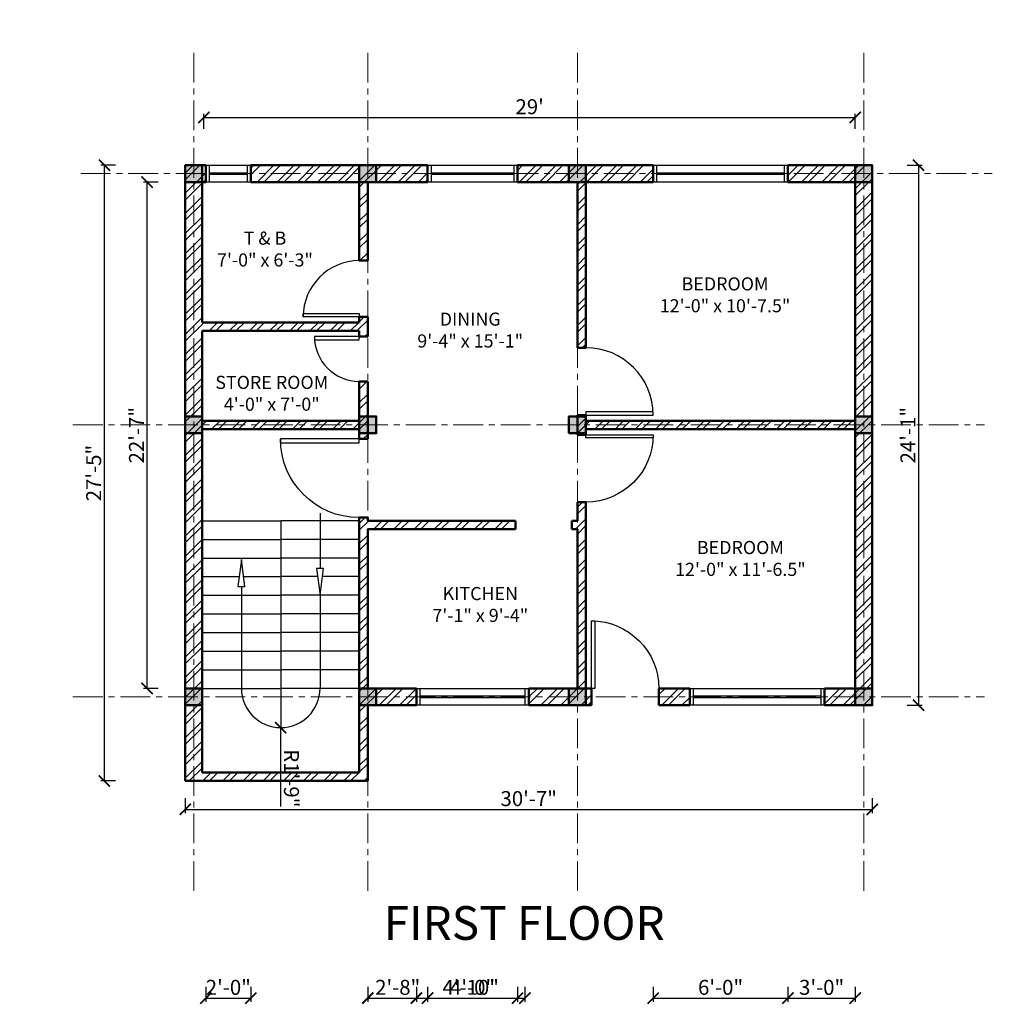
# Model space of a CAD drawing. Units: inches. Extents: x 378 to 1617, y 130 to 1256.
# Tile 4 of 5: x 1028 to 1548, y 134 to 660. Entities that reach past the tile are written whole.
import ezdxf

# ---------------------------------------------------------------- set-up
doc = ezdxf.new("R2010")
doc.units = ezdxf.units.IN
doc.linetypes.add('CENTER', pattern=[50.8, 31.75, -6.35, 6.35, -6.35])
for name, color, linetype, lineweight in [('A-ANNO-TEXT', 7, 'Continuous', 25), ('A-AREA-IDEN', 3, 'Continuous', 18), ('Column Hatch', 1, 'Continuous', 13), ('Columns', 241, 'Continuous', 50), ('Dimensions', 153, 'Continuous', 18), ('Doors', 2, 'Continuous', 25), ('Grid lines', 7, 'CENTER', 18), ('Stairs', 40, 'Continuous', 25), ('Wall Hatch', 11, 'Continuous', 13), ('Walls', 220, 'Continuous', 50), ('Windows', 140, 'Continuous', 25)]:
    doc.layers.add(name, color=color, linetype=linetype, lineweight=lineweight)
doc.styles.get("Standard").update_dxf_attribs({"font": 'arial.ttf'})
doc.dimstyles.new('ISO-25', dxfattribs={"dimtxt": 8, "dimasz": 6, "dimexe": 2, "dimexo": 4, "dimtad": 1, "dimdec": 0, "dimlunit": 3, "dimtxsty": 'Standard', "dimblk": 'ARCHTICK', "dimcen": 2.5, "dimadec": 0, "dimazin": 0, "dimtfac": 1, "dimtdec": 0, "dimtmove": 0, "dimatfit": 3, "dimfxl": 6, "dimfxlon": 1, "dimarcsym": 0})

# ---------------------------------------------------------------- blocks, each defined once
blk = doc.blocks.new('*U3')
for p, q in [((-30, 0), (-30, 4)), ((0, 0), (0, 4))]:
    blk.add_line(p, q)
blk.add_lwpolyline([(0, 0), (0, -30), (-1.75, -30), (-1.75, 0)], close=True)
blk.add_arc((0, 0), 30, 180, 270)
blk = doc.blocks.new('*U4')
for p, q in [((0, 0), (0, 4)), ((24, 0), (24, 4))]:
    blk.add_line(p, q)
blk.add_lwpolyline([(0, 0), (0, -24), (1.75, -24), (1.75, 0)], close=True)
blk.add_arc((0, 0), 24, 270, 0)
blk = doc.blocks.new('*U5')
for p, q in [((0, 0), (0, -4)), ((-36, 0), (-36, -4))]:
    blk.add_line(p, q)
blk.add_lwpolyline([(0, 0), (0, 36), (-1.75, 36), (-1.75, 0)], close=True)
blk.add_arc((0, 0), 36, 90, 180)
blk = doc.blocks.new('*U6')
for p, q in [((0, 0), (0, -4)), ((-36, 0), (-36, -4))]:
    blk.add_line(p, q)
blk.add_lwpolyline([(0, 0), (0, 36), (-1.75, 36), (-1.75, 0)], close=True)
blk.add_arc((0, 0), 36, 90, 180)
blk = doc.blocks.new('*U7')
for p, q in [((-36, 0), (-36, 4)), ((0, 0), (0, 4))]:
    blk.add_line(p, q)
blk.add_lwpolyline([(0, 0), (0, -36), (-1.75, -36), (-1.75, 0)], close=True)
blk.add_arc((0, 0), 36, 180, 270)
blk = doc.blocks.new('_ArchTick')
at = {"color": 0, "linetype": 'ByBlock', "const_width": 0.15}
blk.add_lwpolyline([(-0.5, -0.5), (0.5, 0.5)], dxfattribs=at)
blk = doc.blocks.new('*D39')
at = {"layer": 'Defpoints', "color": 0, "transparency": 16777216}
for p in [(1096.14, 572.95), (1125.53, 572.95), (1125.53, 302.45)]:
    blk.add_point(p, dxfattribs=at)
at = {"layer": 'Dimensions', "color": 0, "lineweight": -2, "transparency": 16777216}
for p, q in [((1102.14, 572.95), (1094.14, 572.95)), ((1096.14, 302.45), (1096.14, 572.95)), ((1102.14, 302.45), (1094.14, 302.45))]:
    blk.add_line(p, q, dxfattribs=at)
at = {"layer": 'Dimensions', "color": 0, "lineweight": -2, "transparency": 16777216, "xscale": 6, "yscale": 6, "zscale": 6}
for p, rotation in [((1096.14, 572.95), 90), ((1096.14, 302.45), 270)]:
    blk.add_blockref('_ArchTick', p, dxfattribs=dict(at, rotation=rotation))
at = {"layer": 'Dimensions', "color": 0, "transparency": 16777216, "insert": (1091.5, 437.7), "char_height": 8, "attachment_point": 5, "rotation": 90}
blk.add_mtext('22\'-7"', dxfattribs=at)
blk = doc.blocks.new('*D40')
at = {"layer": 'Defpoints', "color": 0, "transparency": 16777216}
for p in [(1474.53, 607.45), (1126.53, 572.95), (1474.53, 572.95)]:
    blk.add_point(p, dxfattribs=at)
at = {"layer": 'Dimensions', "color": 0, "lineweight": -2, "transparency": 16777216}
for p, q in [((1126.53, 601.45), (1126.53, 609.45)), ((1126.53, 607.45), (1474.53, 607.45)), ((1474.53, 601.45), (1474.53, 609.45))]:
    blk.add_line(p, q, dxfattribs=at)
at = {"layer": 'Dimensions', "color": 0, "lineweight": -2, "transparency": 16777216, "xscale": 6, "yscale": 6, "zscale": 6, "rotation": 180}
blk.add_blockref('_ArchTick', (1126.53, 607.45), dxfattribs=at)
at = {"layer": 'Dimensions', "color": 0, "lineweight": -2, "transparency": 16777216, "xscale": 6, "yscale": 6, "zscale": 6}
blk.add_blockref('_ArchTick', (1474.53, 607.45), dxfattribs=at)
at = {"layer": 'Dimensions', "color": 0, "transparency": 16777216, "insert": (1300.53, 612.16), "char_height": 8, "attachment_point": 5}
blk.add_mtext("29'", dxfattribs=at)
blk = doc.blocks.new('*D41')
at = {"layer": 'Defpoints', "color": 0, "transparency": 16777216}
for p in [(1483.53, 293.45), (1116.53, 252.95), (1483.53, 237.79)]:
    blk.add_point(p, dxfattribs=at)
at = {"layer": 'Dimensions', "color": 0, "lineweight": -2, "transparency": 16777216}
for p, q in [((1116.53, 243.79), (1116.53, 235.79)), ((1483.53, 243.79), (1483.53, 235.79)), ((1116.53, 237.79), (1483.53, 237.79))]:
    blk.add_line(p, q, dxfattribs=at)
at = {"layer": 'Dimensions', "color": 0, "lineweight": -2, "transparency": 16777216, "xscale": 6, "yscale": 6, "zscale": 6, "rotation": 180}
blk.add_blockref('_ArchTick', (1116.53, 237.79), dxfattribs=at)
at = {"layer": 'Dimensions', "color": 0, "lineweight": -2, "transparency": 16777216, "xscale": 6, "yscale": 6, "zscale": 6}
blk.add_blockref('_ArchTick', (1483.53, 237.79), dxfattribs=at)
at = {"layer": 'Dimensions', "color": 0, "transparency": 16777216, "insert": (1300.03, 242.5), "char_height": 8, "attachment_point": 5}
blk.add_mtext('30\'-7"', dxfattribs=at)
blk = doc.blocks.new('*D42')
at = {"layer": 'Defpoints', "color": 0, "transparency": 16777216}
for p in [(1073.34, 581.95), (1116.53, 581.95), (1116.53, 252.95)]:
    blk.add_point(p, dxfattribs=at)
at = {"layer": 'Dimensions', "color": 0, "lineweight": -2, "transparency": 16777216}
for p, q in [((1079.34, 581.95), (1071.34, 581.95)), ((1073.34, 252.95), (1073.34, 581.95)), ((1079.34, 252.95), (1071.34, 252.95))]:
    blk.add_line(p, q, dxfattribs=at)
at = {"layer": 'Dimensions', "color": 0, "lineweight": -2, "transparency": 16777216, "xscale": 6, "yscale": 6, "zscale": 6}
for p, rotation in [((1073.34, 581.95), 90), ((1073.34, 252.95), 270)]:
    blk.add_blockref('_ArchTick', p, dxfattribs=dict(at, rotation=rotation))
at = {"layer": 'Dimensions', "color": 0, "transparency": 16777216, "insert": (1068.63, 417.45), "char_height": 8, "attachment_point": 5, "rotation": 90}
blk.add_mtext('27\'-5"', dxfattribs=at)
blk = doc.blocks.new('*D43')
at = {"layer": 'Defpoints', "color": 0, "transparency": 16777216}
for p in [(1483.53, 581.95), (1483.53, 293.45), (1508.31, 293.45)]:
    blk.add_point(p, dxfattribs=at)
at = {"layer": 'Dimensions', "color": 0, "lineweight": -2, "transparency": 16777216}
for p, q in [((1502.31, 581.95), (1510.31, 581.95)), ((1508.31, 581.95), (1508.31, 293.45)), ((1502.31, 293.45), (1510.31, 293.45))]:
    blk.add_line(p, q, dxfattribs=at)
at = {"layer": 'Dimensions', "color": 0, "lineweight": -2, "transparency": 16777216, "xscale": 6, "yscale": 6, "zscale": 6}
for p, rotation in [((1508.31, 581.95), 90), ((1508.31, 293.45), 270)]:
    blk.add_blockref('_ArchTick', p, dxfattribs=dict(at, rotation=rotation))
at = {"layer": 'Dimensions', "color": 0, "transparency": 16777216, "insert": (1503.67, 437.7), "char_height": 8, "attachment_point": 5, "rotation": 90}
blk.add_mtext('24\'-1"', dxfattribs=at)
blk = doc.blocks.new('*D65')
at = {"layer": 'Defpoints', "color": 0, "transparency": 16777216}
for p in [(1127.53, 572.95), (1151.53, 572.95), (1151.53, 136.95)]:
    blk.add_point(p, dxfattribs=at)
at = {"layer": 'Dimensions', "color": 0, "lineweight": -2, "transparency": 16777216}
for p, q in [((1127.53, 142.95), (1127.53, 134.95)), ((1151.53, 142.95), (1151.53, 134.95)), ((1127.53, 136.95), (1151.53, 136.95))]:
    blk.add_line(p, q, dxfattribs=at)
at = {"layer": 'Dimensions', "color": 0, "lineweight": -2, "transparency": 16777216, "xscale": 6, "yscale": 6, "zscale": 6, "rotation": 180}
blk.add_blockref('_ArchTick', (1127.53, 136.95), dxfattribs=at)
at = {"layer": 'Dimensions', "color": 0, "lineweight": -2, "transparency": 16777216, "xscale": 6, "yscale": 6, "zscale": 6}
blk.add_blockref('_ArchTick', (1151.53, 136.95), dxfattribs=at)
at = {"layer": 'Dimensions', "color": 0, "transparency": 16777216, "insert": (1139.53, 141.66), "char_height": 8, "attachment_point": 5}
blk.add_mtext('2\'-0"', dxfattribs=at)
blk = doc.blocks.new('*D66')
at = {"layer": 'Defpoints', "color": 0, "transparency": 16777216}
for p in [(1214.03, 572.95), (1246.03, 572.95), (1246.03, 136.95)]:
    blk.add_point(p, dxfattribs=at)
at = {"layer": 'Dimensions', "color": 0, "lineweight": -2, "transparency": 16777216}
for p, q in [((1214.03, 142.95), (1214.03, 134.95)), ((1246.03, 142.95), (1246.03, 134.95)), ((1214.03, 136.95), (1246.03, 136.95))]:
    blk.add_line(p, q, dxfattribs=at)
at = {"layer": 'Dimensions', "color": 0, "lineweight": -2, "transparency": 16777216, "xscale": 6, "yscale": 6, "zscale": 6, "rotation": 180}
blk.add_blockref('_ArchTick', (1214.03, 136.95), dxfattribs=at)
at = {"layer": 'Dimensions', "color": 0, "lineweight": -2, "transparency": 16777216, "xscale": 6, "yscale": 6, "zscale": 6}
blk.add_blockref('_ArchTick', (1246.03, 136.95), dxfattribs=at)
at = {"layer": 'Dimensions', "color": 0, "transparency": 16777216, "insert": (1230.03, 141.66), "char_height": 8, "attachment_point": 5}
blk.add_mtext('2\'-8"', dxfattribs=at)
blk = doc.blocks.new('*D67')
at = {"layer": 'Defpoints', "color": 0, "transparency": 16777216}
for p in [(1246.03, 572.95), (1294.03, 572.95), (1294.03, 136.95)]:
    blk.add_point(p, dxfattribs=at)
at = {"layer": 'Dimensions', "color": 0, "lineweight": -2, "transparency": 16777216}
for p, q in [((1246.03, 142.95), (1246.03, 134.95)), ((1294.03, 142.95), (1294.03, 134.95)), ((1246.03, 136.95), (1294.03, 136.95))]:
    blk.add_line(p, q, dxfattribs=at)
at = {"layer": 'Dimensions', "color": 0, "lineweight": -2, "transparency": 16777216, "xscale": 6, "yscale": 6, "zscale": 6, "rotation": 180}
blk.add_blockref('_ArchTick', (1246.03, 136.95), dxfattribs=at)
at = {"layer": 'Dimensions', "color": 0, "lineweight": -2, "transparency": 16777216, "xscale": 6, "yscale": 6, "zscale": 6}
blk.add_blockref('_ArchTick', (1294.03, 136.95), dxfattribs=at)
at = {"layer": 'Dimensions', "color": 0, "transparency": 16777216, "insert": (1270.03, 141.66), "char_height": 8, "attachment_point": 5}
blk.add_mtext('4\'-0"', dxfattribs=at)
blk = doc.blocks.new('*D68')
at = {"layer": 'Defpoints', "color": 0, "transparency": 16777216}
for p in [(1366.53, 572.95), (1438.53, 572.95), (1438.53, 136.95)]:
    blk.add_point(p, dxfattribs=at)
at = {"layer": 'Dimensions', "color": 0, "lineweight": -2, "transparency": 16777216}
for p, q in [((1366.53, 142.95), (1366.53, 134.95)), ((1438.53, 142.95), (1438.53, 134.95)), ((1366.53, 136.95), (1438.53, 136.95))]:
    blk.add_line(p, q, dxfattribs=at)
at = {"layer": 'Dimensions', "color": 0, "lineweight": -2, "transparency": 16777216, "xscale": 6, "yscale": 6, "zscale": 6, "rotation": 180}
blk.add_blockref('_ArchTick', (1366.53, 136.95), dxfattribs=at)
at = {"layer": 'Dimensions', "color": 0, "lineweight": -2, "transparency": 16777216, "xscale": 6, "yscale": 6, "zscale": 6}
blk.add_blockref('_ArchTick', (1438.53, 136.95), dxfattribs=at)
at = {"layer": 'Dimensions', "color": 0, "transparency": 16777216, "insert": (1402.53, 141.66), "char_height": 8, "attachment_point": 5}
blk.add_mtext('6\'-0"', dxfattribs=at)
blk = doc.blocks.new('*D69')
at = {"layer": 'Defpoints', "color": 0, "transparency": 16777216}
for p in [(1438.53, 572.95), (1474.53, 572.95), (1474.53, 136.95)]:
    blk.add_point(p, dxfattribs=at)
at = {"layer": 'Dimensions', "color": 0, "lineweight": -2, "transparency": 16777216}
for p, q in [((1438.53, 142.95), (1438.53, 134.95)), ((1474.53, 142.95), (1474.53, 134.95)), ((1438.53, 136.95), (1474.53, 136.95))]:
    blk.add_line(p, q, dxfattribs=at)
at = {"layer": 'Dimensions', "color": 0, "lineweight": -2, "transparency": 16777216, "xscale": 6, "yscale": 6, "zscale": 6, "rotation": 180}
blk.add_blockref('_ArchTick', (1438.53, 136.95), dxfattribs=at)
at = {"layer": 'Dimensions', "color": 0, "lineweight": -2, "transparency": 16777216, "xscale": 6, "yscale": 6, "zscale": 6}
blk.add_blockref('_ArchTick', (1474.53, 136.95), dxfattribs=at)
at = {"layer": 'Dimensions', "color": 0, "transparency": 16777216, "insert": (1456.53, 141.66), "char_height": 8, "attachment_point": 5}
blk.add_mtext('3\'-0"', dxfattribs=at)
blk = doc.blocks.new('*D70')
at = {"layer": 'Defpoints', "color": 0, "transparency": 16777216}
for p in [(1240.03, 293.45), (1298.03, 293.45), (1298.03, 136.95)]:
    blk.add_point(p, dxfattribs=at)
at = {"layer": 'Dimensions', "color": 0, "lineweight": -2, "transparency": 16777216}
for p, q in [((1240.03, 142.95), (1240.03, 134.95)), ((1298.03, 142.95), (1298.03, 134.95)), ((1240.03, 136.95), (1298.03, 136.95))]:
    blk.add_line(p, q, dxfattribs=at)
at = {"layer": 'Dimensions', "color": 0, "lineweight": -2, "transparency": 16777216, "xscale": 6, "yscale": 6, "zscale": 6, "rotation": 180}
blk.add_blockref('_ArchTick', (1240.03, 136.95), dxfattribs=at)
at = {"layer": 'Dimensions', "color": 0, "lineweight": -2, "transparency": 16777216, "xscale": 6, "yscale": 6, "zscale": 6}
blk.add_blockref('_ArchTick', (1298.03, 136.95), dxfattribs=at)
at = {"layer": 'Dimensions', "color": 0, "transparency": 16777216, "insert": (1269.03, 141.66), "char_height": 8, "attachment_point": 5}
blk.add_mtext('4\'-10"', dxfattribs=at)
blk = doc.blocks.new('*D71')
at = {"layer": 'Defpoints', "color": 0, "transparency": 16777216}
for p in [(1369.53, 697.95), (1333.53, 302.45), (1369.53, 302.45)]:
    blk.add_point(p, dxfattribs=at)
at = {"layer": 'Dimensions', "color": 0, "lineweight": -2, "transparency": 16777216}
for p, q in [((1333.53, 691.95), (1333.53, 699.95)), ((1369.53, 691.95), (1369.53, 699.95)), ((1333.53, 697.95), (1369.53, 697.95))]:
    blk.add_line(p, q, dxfattribs=at)
at = {"layer": 'Dimensions', "color": 0, "lineweight": -2, "transparency": 16777216, "xscale": 6, "yscale": 6, "zscale": 6, "rotation": 180}
blk.add_blockref('_ArchTick', (1333.53, 697.95), dxfattribs=at)
at = {"layer": 'Dimensions', "color": 0, "lineweight": -2, "transparency": 16777216, "xscale": 6, "yscale": 6, "zscale": 6}
blk.add_blockref('_ArchTick', (1369.53, 697.95), dxfattribs=at)
at = {"layer": 'Dimensions', "color": 0, "transparency": 16777216, "insert": (1351.53, 702.66), "char_height": 8, "attachment_point": 5}
blk.add_mtext('3\'-0"', dxfattribs=at)
blk = doc.blocks.new('*D72')
at = {"layer": 'Defpoints', "color": 0, "transparency": 16777216}
for p in [(1386.03, 697.95), (1369.53, 302.45), (1386.03, 302.45)]:
    blk.add_point(p, dxfattribs=at)
at = {"layer": 'Dimensions', "color": 0, "lineweight": -2, "transparency": 16777216}
for p, q in [((1369.53, 691.95), (1369.53, 699.95)), ((1386.03, 691.95), (1386.03, 699.95)), ((1369.53, 697.95), (1386.03, 697.95)), ((1386.03, 697.95), (1432.43, 697.95))]:
    blk.add_line(p, q, dxfattribs=at)
at = {"layer": 'Dimensions', "color": 0, "lineweight": -2, "transparency": 16777216, "xscale": 6, "yscale": 6, "zscale": 6, "rotation": 180}
blk.add_blockref('_ArchTick', (1369.53, 697.95), dxfattribs=at)
at = {"layer": 'Dimensions', "color": 0, "lineweight": -2, "transparency": 16777216, "xscale": 6, "yscale": 6, "zscale": 6}
blk.add_blockref('_ArchTick', (1386.03, 697.95), dxfattribs=at)
at = {"layer": 'Dimensions', "color": 0, "transparency": 16777216, "insert": (1412.23, 702.71), "char_height": 8, "attachment_point": 5}
blk.add_mtext('1\'-4 1/2"', dxfattribs=at)
blk = doc.blocks.new('*D73')
at = {"layer": 'Defpoints', "color": 0, "transparency": 16777216}
for p in [(1458.03, 697.95), (1386.03, 302.45), (1458.03, 302.45)]:
    blk.add_point(p, dxfattribs=at)
at = {"layer": 'Dimensions', "color": 0, "lineweight": -2, "transparency": 16777216}
for p, q in [((1386.03, 691.95), (1386.03, 699.95)), ((1458.03, 691.95), (1458.03, 699.95)), ((1386.03, 697.95), (1458.03, 697.95))]:
    blk.add_line(p, q, dxfattribs=at)
at = {"layer": 'Dimensions', "color": 0, "lineweight": -2, "transparency": 16777216, "xscale": 6, "yscale": 6, "zscale": 6, "rotation": 180}
blk.add_blockref('_ArchTick', (1386.03, 697.95), dxfattribs=at)
at = {"layer": 'Dimensions', "color": 0, "lineweight": -2, "transparency": 16777216, "xscale": 6, "yscale": 6, "zscale": 6}
blk.add_blockref('_ArchTick', (1458.03, 697.95), dxfattribs=at)
at = {"layer": 'Dimensions', "color": 0, "transparency": 16777216, "insert": (1422.03, 702.66), "char_height": 8, "attachment_point": 5}
blk.add_mtext('6\'-0"', dxfattribs=at)
blk = doc.blocks.new('*D101')
at = {"layer": 'Defpoints', "color": 0, "transparency": 16777216}
for p in [(1167.53, 302.45), (1167.53, 281.45)]:
    blk.add_point(p, dxfattribs=at)
at = {"layer": 'Dimensions', "color": 0, "lineweight": -2, "transparency": 16777216}
for p in [(1167.53, 302.45), (1167.53, 239.28)]:
    blk.add_line(p, (1167.53, 281.45), dxfattribs=at)
at = {"layer": 'Dimensions', "color": 0, "lineweight": -2, "transparency": 16777216, "xscale": 6, "yscale": 6, "zscale": 6, "rotation": 90.00040107045648}
blk.add_blockref('_ArchTick', (1167.53, 281.45), dxfattribs=at)
at = {"layer": 'Dimensions', "color": 0, "transparency": 16777216, "insert": (1172.24, 254.36), "char_height": 8, "attachment_point": 5, "rotation": 270.0004}
blk.add_mtext('R1\'-9"', dxfattribs=at)

msp = doc.modelspace()

# ---------------------------------------------------------------- hatches: boundary and pattern name
at = {"layer": 'Column Hatch'}
h = msp.add_hatch(color=256, dxfattribs=at)
h.dxf.hatch_style = 1
h.paths.add_polyline_path([(525.53, 581.95), (516.53, 581.95), (516.53, 572.95), (525.53, 572.95)])
h.paths.add_polyline_path([(618.53, 581.95), (609.53, 581.95), (609.53, 572.95), (618.53, 572.95)])
h.paths.add_polyline_path([(730.53, 581.95), (721.53, 581.95), (721.53, 572.95), (730.53, 572.95)])
h.paths.add_polyline_path([(883.53, 581.95), (874.53, 581.95), (874.53, 572.95), (883.53, 572.95)])
h.paths.add_polyline_path([(883.53, 447.7), (874.53, 447.7), (874.53, 438.7), (883.53, 438.7)])
h.paths.add_polyline_path([(730.53, 447.7), (721.53, 447.7), (721.53, 438.7), (730.53, 438.7)])
h.paths.add_polyline_path([(618.53, 447.7), (609.53, 447.7), (609.53, 438.7), (618.53, 438.7)])
h.paths.add_polyline_path([(525.53, 447.7), (516.53, 447.7), (516.53, 438.7), (525.53, 438.7)])
h.paths.add_polyline_path([(525.53, 302.45), (516.53, 302.45), (516.53, 293.45), (525.53, 293.45)])
h.paths.add_polyline_path([(618.53, 302.45), (609.53, 302.45), (609.53, 293.45), (618.53, 293.45)])
h.paths.add_polyline_path([(730.53, 302.45), (721.53, 302.45), (721.53, 293.45), (730.53, 293.45)])
h.paths.add_polyline_path([(883.53, 302.45), (874.53, 302.45), (874.53, 293.45), (883.53, 293.45)])
h.paths.add_polyline_path([(1125.53, 302.45), (1116.53, 302.45), (1116.53, 293.45), (1125.53, 293.45)])
h.paths.add_polyline_path([(1218.53, 302.45), (1209.53, 302.45), (1209.53, 293.45), (1218.53, 293.45)])
h.paths.add_polyline_path([(1330.53, 302.45), (1321.53, 302.45), (1321.53, 293.45), (1330.53, 293.45)])
h.paths.add_polyline_path([(1483.53, 302.45), (1474.53, 302.45), (1474.53, 293.45), (1483.53, 293.45)])
h.paths.add_polyline_path([(1483.53, 447.7), (1474.53, 447.7), (1474.53, 438.7), (1483.53, 438.7)])
h.paths.add_polyline_path([(1330.53, 447.7), (1321.53, 447.7), (1321.53, 438.7), (1330.53, 438.7)])
h.paths.add_polyline_path([(1218.53, 447.7), (1209.53, 447.7), (1209.53, 438.7), (1218.53, 438.7)])
h.paths.add_polyline_path([(1125.53, 447.7), (1116.53, 447.7), (1116.53, 438.7), (1125.53, 438.7)])
h.paths.add_polyline_path([(1125.53, 581.95), (1116.53, 581.95), (1116.53, 572.95), (1125.53, 572.95)])
h.paths.add_polyline_path([(1218.53, 581.95), (1209.53, 581.95), (1209.53, 572.95), (1218.53, 572.95)])
h.paths.add_polyline_path([(1330.53, 581.95), (1321.53, 581.95), (1321.53, 572.95), (1330.53, 572.95)])
h.paths.add_polyline_path([(1483.53, 581.95), (1474.53, 581.95), (1474.53, 572.95), (1483.53, 572.95)])
at = {"layer": 'Wall Hatch'}
h = msp.add_hatch(dxfattribs=at)
h.set_pattern_fill('ANSI32', color=256, scale=0.8)
h.paths.add_polyline_path([(1125.53, 440.95), (1209.53, 440.95), (1209.53, 435.7), (1214.03, 435.7), (1214.03, 466.45), (1209.53, 466.45), (1209.53, 445.45), (1125.53, 445.45), (1125.53, 493.45), (1209.53, 493.45), (1209.53, 490.45), (1214.03, 490.45), (1214.03, 500.95), (1209.53, 500.95), (1209.53, 497.95), (1125.53, 497.95), (1125.53, 572.95), (1127.53, 572.95), (1127.53, 581.95), (1116.53, 581.95), (1116.53, 252.95), (1214.03, 252.95), (1214.03, 293.45), (1209.53, 293.45), (1209.53, 257.45), (1125.53, 257.45)])
h.paths.add_polyline_path([(1214.03, 387.45), (1293.03, 387.45), (1293.03, 391.95), (1214.03, 391.95), (1214.03, 393.7), (1209.53, 393.7), (1209.53, 293.45), (1240.03, 293.45), (1240.03, 302.45), (1214.03, 302.45)])
h.paths.add_polyline_path([(1333.53, 302.45), (1330.53, 302.45), (1330.53, 401.95), (1326.03, 401.95), (1326.03, 391.95), (1323.03, 391.95), (1323.03, 387.45), (1326.03, 387.45), (1326.03, 302.45), (1300.03, 302.45), (1300.03, 293.45), (1333.53, 293.45)])
h.paths.add_polyline_path([(1386.03, 302.45), (1369.53, 302.45), (1369.53, 293.45), (1386.03, 293.45)], flags=17)
h.paths.add_polyline_path([(1483.53, 581.95), (1438.53, 581.95), (1438.53, 572.95), (1474.53, 572.95), (1474.53, 445.45), (1330.53, 445.45), (1330.53, 448.45), (1326.03, 448.45), (1326.03, 437.95), (1330.53, 437.95), (1330.53, 440.95), (1474.53, 440.95), (1474.53, 302.45), (1458.03, 302.45), (1458.03, 293.45), (1483.53, 293.45)])
h.paths.add_polyline_path([(1330.53, 572.95), (1366.53, 572.95), (1366.53, 581.95), (1294.03, 581.95), (1294.03, 572.95), (1326.03, 572.95), (1326.03, 484.45), (1330.53, 484.45)])
h.paths.add_polyline_path([(1246.03, 581.95), (1151.53, 581.95), (1151.53, 572.95), (1209.53, 572.95), (1209.53, 530.95), (1214.03, 530.95), (1214.03, 572.95), (1246.03, 572.95)])

# ---------------------------------------------------------------- linework, layer by layer
at = {"layer": 'Columns'}
for points in [[(1116.53, 572.95), (1125.53, 572.95), (1125.53, 581.95), (1116.53, 581.95)], [(1209.53, 572.95), (1218.53, 572.95), (1218.53, 581.95), (1209.53, 581.95)], [(1321.53, 572.95), (1330.53, 572.95), (1330.53, 581.95), (1321.53, 581.95)], [(1474.53, 572.95), (1483.53, 572.95), (1483.53, 581.95), (1474.53, 581.95)], [(1116.53, 438.7), (1125.53, 438.7), (1125.53, 447.7), (1116.53, 447.7)], [(1209.53, 438.7), (1218.53, 438.7), (1218.53, 447.7), (1209.53, 447.7)], [(1321.53, 438.7), (1330.53, 438.7), (1330.53, 447.7), (1321.53, 447.7)], [(1474.53, 438.7), (1483.53, 438.7), (1483.53, 447.7), (1474.53, 447.7)], [(1116.53, 293.45), (1125.53, 293.45), (1125.53, 302.45), (1116.53, 302.45)], [(1209.53, 293.45), (1218.53, 293.45), (1218.53, 302.45), (1209.53, 302.45)], [(1321.53, 293.45), (1330.53, 293.45), (1330.53, 302.45), (1321.53, 302.45)], [(1474.53, 293.45), (1483.53, 293.45), (1483.53, 302.45), (1474.53, 302.45)]]:
    msp.add_lwpolyline(points, close=True, dxfattribs=at)
at = {"layer": 'Grid lines', "ltscale": 0.5}
for p, q in [((1121.03, 641.95), (1121.03, 192.95)), ((1214.03, 641.95), (1214.03, 192.95)), ((1326.03, 641.95), (1326.03, 192.95)), ((1479.03, 641.95), (1479.03, 192.95)), ((1060.71, 577.45), (1547.71, 577.45)), ((1056.53, 443.2), (1543.53, 443.2)), ((1056.53, 297.95), (1543.53, 297.95))]:
    msp.add_line(p, q, dxfattribs=at)
at = {"layer": 'Stairs'}
for p, q in [((1188.53, 395.95), (1188.53, 366.47)), ((1125.53, 391.95), (1167.53, 391.95)), ((1209.53, 391.95), (1167.53, 391.95)), ((1167.53, 391.95), (1167.53, 302.45)), ((1209.53, 391.95), (1209.53, 302.45)), ((1125.53, 382.01), (1167.53, 382.01)), ((1209.53, 382.01), (1167.53, 382.01)), ((1125.53, 372.06), (1167.53, 372.06)), ((1209.53, 372.06), (1167.53, 372.06)), ((1125.53, 362.12), (1145.32, 362.12)), ((1147.74, 362.12), (1167.53, 362.12)), ((1187.2, 362.12), (1167.53, 362.12)), ((1209.53, 362.12), (1189.85, 362.12)), ((1146.53, 356.94), (1146.53, 302.45)), ((1125.53, 352.17), (1167.53, 352.17)), ((1209.53, 352.17), (1167.53, 352.17)), ((1188.53, 352.17), (1188.53, 302.45)), ((1125.53, 342.23), (1167.53, 342.23)), ((1209.53, 342.23), (1167.53, 342.23)), ((1125.53, 332.28), (1167.53, 332.28)), ((1209.53, 332.28), (1167.53, 332.28)), ((1125.53, 322.34), (1167.53, 322.34)), ((1209.53, 322.34), (1167.53, 322.34)), ((1125.53, 312.4), (1167.53, 312.4)), ((1209.53, 312.4), (1167.53, 312.4)), ((1125.53, 302.45), (1167.53, 302.45)), ((1209.53, 302.45), (1167.53, 302.45))]:
    msp.add_line(p, q, dxfattribs=at)
for points in [[(1148.43, 356.94), (1146.53, 371.23), (1144.63, 356.94)], [(1186.63, 366.47), (1188.53, 352.17), (1190.43, 366.47)]]:
    msp.add_lwpolyline(points, close=True, dxfattribs=at)
msp.add_arc((1167.53, 302.45), 21, 180, 0, dxfattribs=at)
at = {"layer": 'Walls'}
for p, q in [((1116.53, 252.95), (1116.53, 581.95)), ((1116.53, 581.95), (1127.53, 581.95)), ((1127.53, 581.95), (1127.53, 572.95)), ((1151.53, 581.95), (1246.03, 581.95)), ((1151.53, 581.95), (1151.53, 572.95)), ((1246.03, 572.95), (1246.03, 581.95)), ((1294.03, 581.95), (1366.53, 581.95)), ((1294.03, 572.95), (1294.03, 581.95)), ((1366.53, 572.95), (1366.53, 581.95)), ((1438.53, 581.95), (1483.53, 581.95)), ((1438.53, 572.95), (1438.53, 581.95)), ((1483.53, 581.95), (1483.53, 293.45)), ((1125.53, 497.95), (1125.53, 572.95)), ((1125.53, 572.95), (1127.53, 572.95)), ((1151.53, 572.95), (1209.53, 572.95)), ((1209.53, 572.95), (1209.53, 530.95)), ((1214.03, 572.95), (1214.03, 530.95)), ((1214.03, 572.95), (1246.03, 572.95)), ((1294.03, 572.95), (1326.03, 572.95)), ((1326.03, 572.95), (1326.03, 484.45)), ((1330.53, 572.95), (1330.53, 484.45)), ((1330.53, 572.95), (1366.53, 572.95)), ((1438.53, 572.95), (1474.53, 572.95)), ((1474.53, 572.95), (1474.53, 445.45)), ((1209.53, 530.95), (1214.03, 530.95)), ((1209.53, 500.95), (1209.53, 497.95)), ((1209.53, 500.95), (1214.03, 500.95)), ((1214.03, 500.95), (1214.03, 490.45)), ((1209.53, 497.95), (1125.53, 497.95)), ((1209.53, 493.45), (1125.53, 493.45)), ((1125.53, 493.45), (1125.53, 445.45)), ((1209.53, 493.45), (1209.53, 490.45)), ((1209.53, 490.45), (1214.03, 490.45)), ((1330.53, 484.45), (1326.03, 484.45)), ((1209.53, 466.45), (1209.53, 445.45)), ((1209.53, 466.45), (1214.03, 466.45)), ((1214.03, 466.45), (1214.03, 435.7)), ((1326.03, 448.45), (1326.03, 437.95)), ((1330.53, 448.45), (1326.03, 448.45)), ((1330.53, 448.45), (1330.53, 445.45)), ((1209.53, 445.45), (1125.53, 445.45)), ((1330.53, 445.45), (1474.53, 445.45)), ((1209.53, 440.95), (1125.53, 440.95)), ((1125.53, 440.95), (1125.53, 257.45)), ((1209.53, 440.95), (1209.53, 435.7)), ((1330.53, 437.95), (1326.03, 437.95)), ((1330.53, 440.95), (1330.53, 437.95)), ((1330.53, 440.95), (1474.53, 440.95)), ((1474.53, 440.95), (1474.53, 302.45)), ((1209.53, 435.7), (1214.03, 435.7)), ((1326.03, 401.95), (1326.03, 391.95)), ((1330.53, 401.95), (1326.03, 401.95)), ((1330.53, 401.95), (1330.53, 302.45)), ((1209.53, 393.7), (1209.53, 257.45)), ((1209.53, 393.7), (1214.03, 393.7)), ((1214.03, 393.7), (1214.03, 391.95)), ((1214.03, 391.95), (1293.03, 391.95)), ((1293.03, 391.95), (1293.03, 387.45)), ((1323.03, 391.95), (1326.03, 391.95)), ((1323.03, 391.95), (1323.03, 387.45)), ((1214.03, 387.45), (1293.03, 387.45)), ((1214.03, 387.45), (1214.03, 302.45)), ((1323.03, 387.45), (1326.03, 387.45)), ((1326.03, 387.45), (1326.03, 302.45)), ((1214.03, 302.45), (1240.03, 302.45)), ((1240.03, 302.45), (1240.03, 293.45)), ((1300.03, 302.45), (1326.03, 302.45)), ((1300.03, 302.45), (1300.03, 293.45)), ((1330.53, 302.45), (1333.53, 302.45)), ((1333.53, 302.45), (1333.53, 293.45)), ((1369.53, 302.45), (1386.03, 302.45)), ((1369.53, 302.45), (1369.53, 293.45)), ((1386.03, 302.45), (1386.03, 293.45)), ((1458.03, 302.45), (1474.53, 302.45)), ((1458.03, 302.45), (1458.03, 293.45)), ((1209.53, 293.45), (1240.03, 293.45)), ((1214.03, 293.45), (1214.03, 252.95)), ((1300.03, 293.45), (1333.53, 293.45)), ((1369.53, 293.45), (1386.03, 293.45)), ((1458.03, 293.45), (1483.53, 293.45)), ((1214.03, 252.95), (1116.53, 252.95)), ((1209.53, 257.45), (1125.53, 257.45))]:
    msp.add_line(p, q, dxfattribs=at)
at = {"layer": 'Windows'}
for p, q in [((1127.53, 572.95), (1127.53, 581.95)), ((1127.53, 581.95), (1151.53, 581.95)), ((1129.53, 572.95), (1129.53, 581.95)), ((1149.53, 581.95), (1149.53, 572.95)), ((1151.53, 581.95), (1151.53, 572.95)), ((1246.03, 572.95), (1246.03, 581.95)), ((1246.03, 581.95), (1294.03, 581.95)), ((1248.03, 572.95), (1248.03, 581.95)), ((1292.03, 581.95), (1292.03, 572.95)), ((1294.03, 581.95), (1294.03, 572.95)), ((1366.53, 572.95), (1366.53, 581.95)), ((1366.53, 581.95), (1438.53, 581.95)), ((1368.53, 572.95), (1368.53, 581.95)), ((1436.53, 581.95), (1436.53, 572.95)), ((1438.53, 581.95), (1438.53, 572.95)), ((1129.53, 577.95), (1149.53, 577.95)), ((1149.53, 576.95), (1129.53, 576.95)), ((1248.03, 577.95), (1292.03, 577.95)), ((1292.03, 576.95), (1248.03, 576.95)), ((1368.53, 577.95), (1436.53, 577.95)), ((1436.53, 576.95), (1368.53, 576.95)), ((1151.53, 572.95), (1127.53, 572.95)), ((1294.03, 572.95), (1246.03, 572.95)), ((1438.53, 572.95), (1366.53, 572.95)), ((1240.03, 302.45), (1300.03, 302.45)), ((1240.03, 293.45), (1240.03, 302.45)), ((1242.03, 293.45), (1242.03, 302.45)), ((1298.03, 302.45), (1298.03, 293.45)), ((1300.03, 302.45), (1300.03, 293.45)), ((1386.03, 293.45), (1386.03, 302.45)), ((1386.03, 302.45), (1458.03, 302.45)), ((1388.03, 293.45), (1388.03, 302.45)), ((1456.03, 302.45), (1456.03, 293.45)), ((1458.03, 302.45), (1458.03, 293.45)), ((1242.03, 298.45), (1298.03, 298.45)), ((1298.03, 297.45), (1242.03, 297.45)), ((1388.03, 298.45), (1456.03, 298.45)), ((1456.03, 297.45), (1388.03, 297.45)), ((1300.03, 293.45), (1240.03, 293.45)), ((1458.03, 293.45), (1386.03, 293.45))]:
    msp.add_line(p, q, dxfattribs=at)

# ---------------------------------------------------------------- block references
at = {"layer": 'Doors', "rotation": 270}
for name, p in [('*U3', (1209.53, 500.95)), ('*U4', (1209.53, 490.45)), ('*U5', (1330.53, 448.45))]:
    msp.add_blockref(name, p, dxfattribs=at)
at = {"layer": 'Doors', "xscale": -1}
for name, p, rotation in [('*U5', (1330.53, 437.95), 269.9999999999999), ('*U6', (1333.53, 302.45), 359.9999999999999)]:
    msp.add_blockref(name, p, dxfattribs=dict(at, rotation=rotation))
at = {"layer": 'Doors', "xscale": -1.166666666666666, "yscale": 1.166666666666666, "zscale": 1.166666666666666, "rotation": 269.9999999999999}
msp.add_blockref('*U7', (1209.36, 435.7), dxfattribs=at)

# ---------------------------------------------------------------- texts
at = {"layer": 'A-ANNO-TEXT', "insert": (1124.62, 186.07), "char_height": 18, "attachment_point": 1}
msp.add_mtext_dynamic_manual_height_columns('\\pxqc;{\\fTimes New Roman|b0|i0|c0|p18;FIRST FLOOR}', width=345.962, gutter_width=12.5, heights=[0], dxfattribs=at)
at = {"layer": 'A-AREA-IDEN', "char_height": 7, "attachment_point": 1}
for s, width, insert in [('\\pxqc;{\\fTimes New Roman|b0|i0|c0|p18;T & B\\P7\'-0" x 6\'-3"}', 57.8149, (1130.2, 546.48)), ('\\pxqc;{\\fTimes New Roman|b0|i0|c0|p18;BEDROOM\\P12\'-0" x 10\'-7.5"}', 73.2905, (1368.28, 522.03)), ('\\pxqc;{\\fTimes New Roman|b0|i0|c0|p18;DINING\\P9\'-4" x 15\'-1"}', 57.8149, (1239.86, 503.21)), ('\\pxqc;{\\fTimes New Roman|b0|i0|c0|p18;STORE ROOM\\P4\'-0" x 7\'-0"}', 67.3594, (1129.07, 469.41)), ('\\pxqc;{\\fTimes New Roman|b0|i0|c0|p18;BEDROOM\\P12\'-0" x 11\'-6.5"}', 70.4926, (1377.89, 381.18)), ('\\pxqc;{\\fTimes New Roman|b0|i0|c0|p18;KITCHEN\\P7\'-1" x 9\'-4"}', 57.8149, (1245.27, 356.58))]:
    msp.add_mtext_dynamic_manual_height_columns(s, width=width, gutter_width=12.5, heights=[0], dxfattribs=dict(at, insert=insert))

# ---------------------------------------------------------------- dimensions: what is measured, and where the dimension line sits
at = {"layer": 'Dimensions'}
for base, p1, p2, override, picture, middle in [((1386.03, 697.95), (1369.53, 302.45), (1386.03, 302.45), {"dimdec": 1, "dimlfac": 1, "dimrnd": 0, "dimzin": 1, "dimdsep": 46, "dimlunit": 4, "dimfrac": 2}, '*D72', (1412.23, 702.71)), ((1369.53, 697.95), (1333.53, 302.45), (1369.53, 302.45), {"dimdec": 1, "dimlfac": 1, "dimrnd": 0, "dimzin": 1, "dimdsep": 46, "dimlunit": 4, "dimfrac": 2}, '*D71', (1351.53, 702.66)), ((1458.03, 697.95), (1386.03, 302.45), (1458.03, 302.45), {"dimdec": 1, "dimlfac": 1, "dimrnd": 0, "dimzin": 1, "dimdsep": 46, "dimlunit": 4, "dimfrac": 2}, '*D73', (1422.03, 702.66)), ((1474.53, 607.45), (1126.53, 572.95), (1474.53, 572.95), {"dimclrd": 0, "dimclre": 0, "dimclrt": 0}, '*D40', (1300.53, 612.16)), ((1151.53, 136.95), (1127.53, 572.95), (1151.53, 572.95), {"dimdec": 1, "dimlfac": 1, "dimrnd": 0, "dimzin": 1, "dimdsep": 46, "dimlunit": 4, "dimfrac": 2}, '*D65', (1139.53, 141.66)), ((1246.03, 136.95), (1214.03, 572.95), (1246.03, 572.95), {"dimdec": 1, "dimlfac": 1, "dimrnd": 0, "dimzin": 1, "dimdsep": 46, "dimlunit": 4, "dimfrac": 2}, '*D66', (1230.03, 141.66)), ((1294.03, 136.95), (1246.03, 572.95), (1294.03, 572.95), {"dimdec": 1, "dimlfac": 1, "dimrnd": 0, "dimzin": 1, "dimdsep": 46, "dimlunit": 4, "dimfrac": 2}, '*D67', (1270.03, 141.66)), ((1438.53, 136.95), (1366.53, 572.95), (1438.53, 572.95), {"dimdec": 1, "dimlfac": 1, "dimrnd": 0, "dimzin": 1, "dimdsep": 46, "dimlunit": 4, "dimfrac": 2}, '*D68', (1402.53, 141.66)), ((1474.53, 136.95), (1438.53, 572.95), (1474.53, 572.95), {"dimdec": 1, "dimlfac": 1, "dimrnd": 0, "dimzin": 1, "dimdsep": 46, "dimlunit": 4, "dimfrac": 2}, '*D69', (1456.53, 141.66)), ((1483.53, 237.79), (1116.53, 252.95), (1483.53, 293.45), {"dimclrd": 0, "dimclre": 0, "dimclrt": 0}, '*D41', (1300.03, 242.5)), ((1298.03, 136.95), (1240.03, 293.45), (1298.03, 293.45), {"dimdec": 1, "dimlfac": 1, "dimrnd": 0, "dimzin": 1, "dimdsep": 46, "dimlunit": 4, "dimfrac": 2}, '*D70', (1269.03, 141.66))]:
    dim = msp.add_linear_dim(base=base, p1=p1, p2=p2, dimstyle='ISO-25', override=override, dxfattribs=at)
    dim.commit()
    dim.dimension.update_dxf_attribs({"geometry": picture, "text_midpoint": middle})
for base, p1, p2, picture, middle in [((1073.34, 581.95), (1116.53, 252.95), (1116.53, 581.95), '*D42', (1068.63, 417.45)), ((1508.31443733, 293.45088562), (1483.5278532, 581.95088562), (1483.5278532, 293.45088562), '*D43', (1503.67306626, 437.70088562)), ((1096.1441612, 572.95088562), (1125.5278532, 302.45088562), (1125.5278532, 572.95088562), '*D39', (1091.50279012, 437.70088562))]:
    dim = msp.add_linear_dim(base=base, p1=p1, p2=p2, angle=90, dimstyle='ISO-25', override={"dimclrd": 0, "dimclre": 0, "dimclrt": 0}, dxfattribs=at)
    dim.commit()
    dim.dimension.update_dxf_attribs({"geometry": picture, "text_midpoint": middle})
dim = msp.add_radius_dim(center=(1167.53, 302.45), mpoint=(1167.53, 281.45), dimstyle='ISO-25', override={"dimdec": 1, "dimlfac": 1, "dimrnd": 0, "dimzin": 1, "dimdsep": 46, "dimlunit": 4, "dimfrac": 2}, dxfattribs=at)
dim.commit()
dim.dimension.update_dxf_attribs({"geometry": '*D101', "text_midpoint": (1172.24, 254.36)})

doc.saveas('drawing.dxf')
